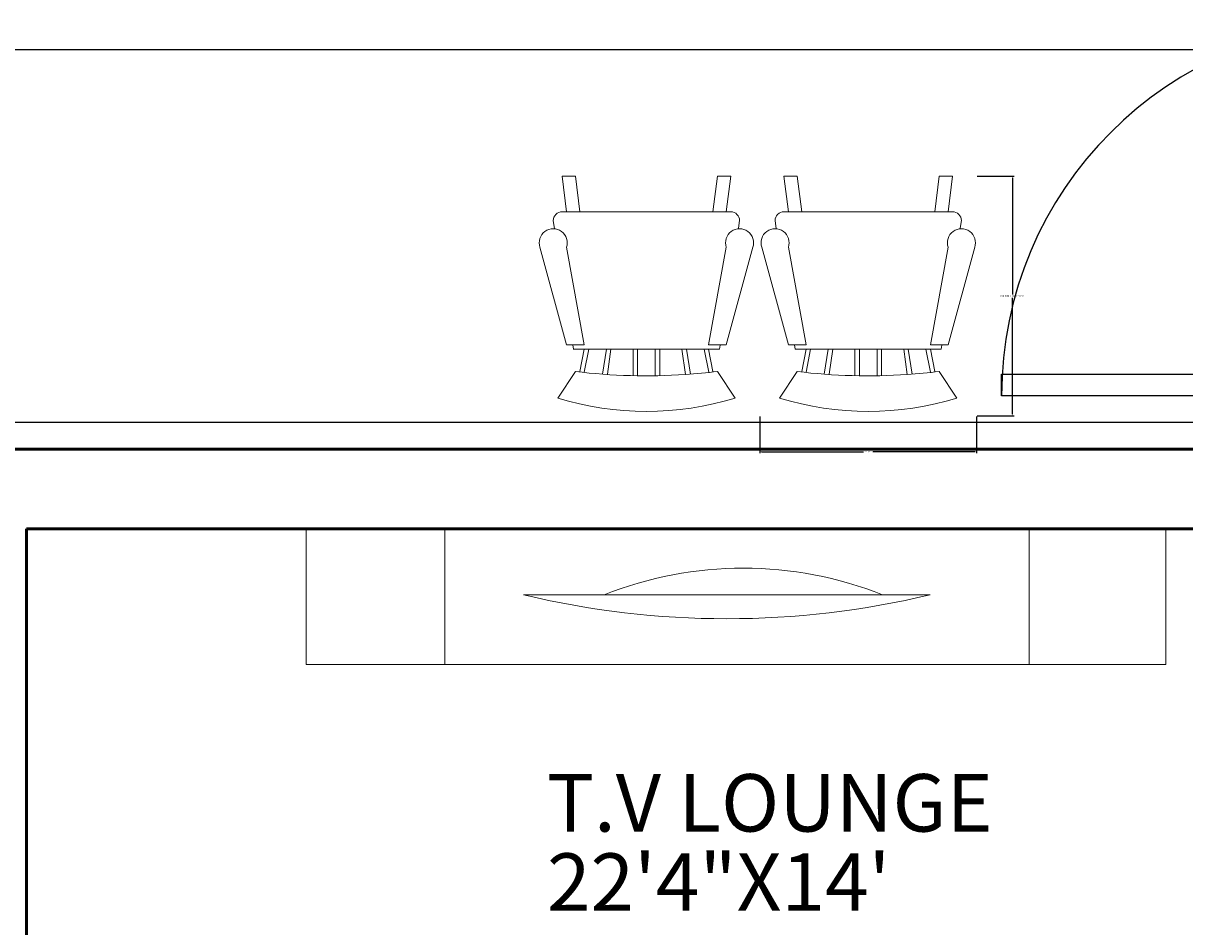
# Model space of a CAD drawing. Units: inches. Extents: x 5375 to 6084, y 16106 to 17259.
# Tile 23 of 32: x 5553 to 5684, y 16823 to 16925. Entities that reach past the tile are written whole.
import ezdxf

# ---------------------------------------------------------------- set-up
doc = ezdxf.new("R2010")
doc.units = ezdxf.units.IN
for name, color, linetype, lineweight in [('A-ANNO-DIMS', 2, 'Continuous', 18), ('A-AREA-IDEN', 5, 'Continuous', 18), ('DOOR', 4, 'Continuous', 25), ('FURNITURE', 3, 'Continuous', 18), ('WALL', 6, 'Continuous', 50)]:
    doc.layers.add(name, color=color, linetype=linetype, lineweight=lineweight)
doc.styles.get("Standard").update_dxf_attribs({"font": 'arial.ttf'})
doc.dimstyles.get("Standard").update_dxf_attribs({"dimtxt": 0.18, "dimasz": 0.18, "dimexe": 0.18, "dimexo": 0.0625, "dimgap": 0.09, "dimtad": 0, "dimtih": 1, "dimtoh": 1, "dimdec": 4, "dimzin": 0, "dimdsep": 46, "dimtxsty": 'Standard', "dimcen": 0.09, "dimadec": 0, "dimazin": 0, "dimtfac": 1, "dimtdec": 4, "dimtofl": 0, "dimtmove": 0, "dimatfit": 3, "dimfxl": 1, "dimtolj": 1, "dimtzin": 0, "dimarcsym": 0})

# ---------------------------------------------------------------- blocks, each defined once
blk = doc.blocks.new('*U2')
for p, q in [((0, 0), (0, -100)), ((750, 0), (750, -100))]:
    blk.add_line(p, q)
blk.add_lwpolyline([(0, 0), (0, 750), (43.75, 750), (43.75, 0)], close=True)
blk.add_arc((0, 0), 750, 0, 90)
blk = doc.blocks.new('Chair - Rocking')
for p, q in [((-8, -4.5), (-10, -1.5)), ((8, -4.5), (10, -1.5)), ((-7.5, -4.5), (-7, -7)), ((-6.5, -7), (-7.02225, -4.43)), ((-4.5, -7), (-4.96674, -4.19951)), ((-4, -7), (-4.40532, -4.16272)), ((-1.5, -4.05012), (-1.5, -7)), ((-1, -7), (-1, -4.05012)), ((1, -7), (1, -4.04655)), ((1.5, -4.05012), (1.5, -7)), ((4, -7), (4.40187, -4.18694)), ((4.5, -7), (4.96761, -4.19437)), ((6.5, -7), (7, -4.4057)), ((7.5, -4.5), (7, -7)), ((-9, -7.5), (-12, -18.49999)), ((-7, -7.5), (-9, -7.5)), ((-9, -18.49999), (-7, -7.5)), ((-8.23428, -6.99939), (-8.3093, -7.47958)), ((-8.23041, -7), (8.23915, -7)), ((7, -7.5), (9, -7.5)), ((9, -18.49999), (7, -7.5)), ((8.31071, -7.48854), (8.23449, -7.00073)), ((9, -7.5), (12, -18.49999)), ((-10.36644, -20.64523), (-10.5, -21.49999)), ((10.5, -21.49999), (10.3575, -20.58798)), ((-9, -22.49999), (-9.5, -26.49999)), ((0, -22.49999), (-9.5, -22.49999)), ((-8, -26.49999), (-7.5, -22.49999)), ((0, -22.49999), (9.5, -22.49999)), ((8, -26.49999), (7.5, -22.49999)), ((9, -22.49999), (9.5, -26.49999)), ((-9.5, -26.49999), (-8, -26.49999)), ((9.5, -26.49999), (8, -26.49999))]:
    blk.add_line(p, q)
for centre, radius, start, end in [((0, -34.08333), 34.08333, 72.93847, 107.0615), ((0, -68.25004), 64.25, 93.92211, 97.15267), ((0, -68.25004), 64.25, 82.84733, 93.92211), ((-10.5, -18.99999), 1.58114, 161.5651, 18.43495), ((10.5, -18.99999), 1.58114, 161.5651, 18.43495), ((-9.5, -21.49999), 1, 180, 270), ((9.5, -21.49999), 1, 270, 0)]:
    blk.add_arc(centre, radius, start, end)
blk = doc.blocks.new('*D22')
at = {"layer": 'A-ANNO-DIMS', "color": 0, "lineweight": -2, "transparency": 16777216}
for p, q in [((5660.78, 16907.33), (5664.94, 16907.33)), ((5664.76, 16907.15), (5664.76, 16894.01)), ((5664.76, 16880.51), (5664.76, 16893.64)), ((5660.78, 16880.33), (5664.94, 16880.33))]:
    blk.add_line(p, q, dxfattribs=at)
at = {"layer": 'A-ANNO-DIMS', "color": 0, "transparency": 16777216}
for points in [[(5664.73, 16907.15), (5664.79, 16907.15), (5664.76, 16907.33)], [(5664.73, 16880.51), (5664.79, 16880.51), (5664.76, 16880.33)]]:
    blk.add_solid(points, dxfattribs=at)
at = {"layer": 'Defpoints', "color": 0, "transparency": 16777216}
for p in [(5660.71, 16907.33), (5660.71, 16880.33), (5664.76, 16880.33)]:
    blk.add_point(p, dxfattribs=at)
at = {"layer": 'A-ANNO-DIMS', "color": 0, "transparency": 16777216, "insert": (5664.76, 16893.83), "char_height": 0.18, "attachment_point": 5}
blk.add_mtext('\\A1;ROCKING CHAIR 27 TYP.', dxfattribs=at)
blk = doc.blocks.new('*D23')
at = {"layer": 'A-ANNO-DIMS', "color": 0, "lineweight": -2, "transparency": 16777216}
for p, q in [((5636.28, 16880.26), (5636.28, 16876.1)), ((5660.71, 16880.26), (5660.71, 16876.1)), ((5636.46, 16876.28), (5647.97, 16876.28)), ((5660.53, 16876.28), (5649.03, 16876.28))]:
    blk.add_line(p, q, dxfattribs=at)
at = {"layer": 'A-ANNO-DIMS', "color": 0, "transparency": 16777216}
for points in [[(5636.46, 16876.31), (5636.46, 16876.25), (5636.28, 16876.28)], [(5660.53, 16876.31), (5660.53, 16876.25), (5660.71, 16876.28)]]:
    blk.add_solid(points, dxfattribs=at)
at = {"layer": 'Defpoints', "color": 0, "transparency": 16777216}
for p in [(5636.28, 16880.33), (5660.71, 16880.33), (5636.28, 16876.28)]:
    blk.add_point(p, dxfattribs=at)
at = {"layer": 'A-ANNO-DIMS', "color": 0, "transparency": 16777216, "insert": (5648.5, 16876.28), "char_height": 0.18, "attachment_point": 5}
blk.add_mtext('\\A1;24 TYP.', dxfattribs=at)
blk = doc.blocks.new('*D42')
at = {"layer": 'A-ANNO-DIMS', "color": 0, "lineweight": -2, "transparency": 16777216}
for p, q in [((5826.06, 16921.58), (5375.56, 16921.58)), ((5375.74, 16921.4), (5375.74, 16900.76)), ((5375.74, 16879.76), (5375.74, 16900.4)), ((5826.06, 16879.58), (5375.56, 16879.58))]:
    blk.add_line(p, q, dxfattribs=at)
at = {"layer": 'A-ANNO-DIMS', "color": 0, "transparency": 16777216}
for points in [[(5375.71, 16921.4), (5375.77, 16921.4), (5375.74, 16921.58)], [(5375.71, 16879.76), (5375.77, 16879.76), (5375.74, 16879.58)]]:
    blk.add_solid(points, dxfattribs=at)
at = {"layer": 'Defpoints', "color": 0, "transparency": 16777216}
for p in [(5826.12, 16921.58), (5375.74, 16879.58), (5826.12, 16879.58)]:
    blk.add_point(p, dxfattribs=at)
at = {"layer": 'A-ANNO-DIMS', "color": 0, "transparency": 16777216, "insert": (5375.74, 16900.58), "char_height": 0.18, "attachment_point": 5}
blk.add_mtext('\\A1;42', dxfattribs=at)

msp = doc.modelspace()

# ---------------------------------------------------------------- linework, layer by layer
at = {"layer": 'FURNITURE'}
for p, q in [((5600.7891, 16867.5793), (5600.7891, 16852.2928)), ((5666.6219, 16867.5793), (5666.6219, 16852.2928)), ((5609.6276, 16860.1564), (5655.4818, 16860.1564))]:
    msp.add_line(p, q, dxfattribs=at)
msp.add_lwpolyline([(5585.1383, 16867.5793), (5682.0242, 16867.5793), (5682.0242, 16852.2928), (5585.1383, 16852.2928)], close=True, dxfattribs=at)
for centre, radius, start, end in [((5634.4279, 16820.655), 42.5035, 68.336249, 111.663751), ((5632.5547, 16955.9552), 98.5041, 256.540815, 283.459185)]:
    msp.add_arc(centre, radius, start, end, dxfattribs=at)
at = {"layer": 'WALL'}
for p, q in [((5529.6199, 16876.5793), (5702.1199, 16876.5793)), ((5553.6199, 16867.5793), (5553.6199, 16699.5793)), ((5553.6199, 16867.5793), (5711.1199, 16867.5793))]:
    msp.add_line(p, q, dxfattribs=at)

# ---------------------------------------------------------------- block references
at = {"layer": 'DOOR', "xscale": 0.0559999999999998, "yscale": 0.0559999999999998, "zscale": 0.0559999999999998, "rotation": 90.00000000000003}
msp.add_blockref('*U2', (5705.5199, 16882.5793), dxfattribs=at)
at = {"layer": 'FURNITURE', "rotation": 180}
for p in [(5623.4981, 16880.8255), (5648.4959, 16880.8255)]:
    msp.add_blockref('Chair - Rocking', p, dxfattribs=at)

# ---------------------------------------------------------------- texts
at = {"layer": 'A-AREA-IDEN'}
for s, p in [('T.V LOUNGE', (5612.2945, 16833.4578)), ('22\'4"X14\'', (5612.2945, 16824.5247))]:
    msp.add_text(s, height=6.47981, dxfattribs=at).set_placement(p)

# ---------------------------------------------------------------- dimensions: what is measured, and where the dimension line sits
at = {"layer": 'A-ANNO-DIMS'}
dim = msp.add_linear_dim(base=(5375.7423, 16879.5793), p1=(5826.1199, 16921.5793), p2=(5826.1199, 16879.5793), angle=90, dimstyle='Standard', override={"dimdec": 0, "dimlfac": 1, "dimrnd": 0, "dimzin": 0, "dimdsep": 46, "dimlunit": 2}, dxfattribs=at)
dim.commit()
dim.dimension.update_dxf_attribs({"geometry": '*D42', "text_midpoint": (5375.7423, 16900.5793)})
for base, p1, p2, angle, text, picture, middle in [((5664.7634, 16880.3255), (5660.7134, 16907.3255), (5660.7134, 16880.3255), 270, 'ROCKING CHAIR <> TYP.', '*D22', (5664.7634, 16893.8255)), ((5636.2783, 16876.2755), (5660.7134, 16880.3255), (5636.2783, 16880.3255), 180, '<> TYP.', '*D23', (5648.4959, 16876.2755))]:
    dim = msp.add_linear_dim(base=base, p1=p1, p2=p2, angle=angle, text=text, dimstyle='Standard', override={"dimdec": 0, "dimlfac": 1, "dimrnd": 0, "dimzin": 0, "dimdsep": 46, "dimlunit": 2}, dxfattribs=at)
    dim.commit()
    dim.dimension.update_dxf_attribs({"geometry": picture, "text_midpoint": middle})

doc.saveas('drawing.dxf')
